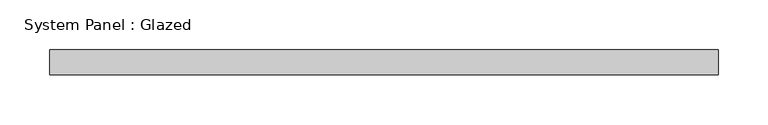
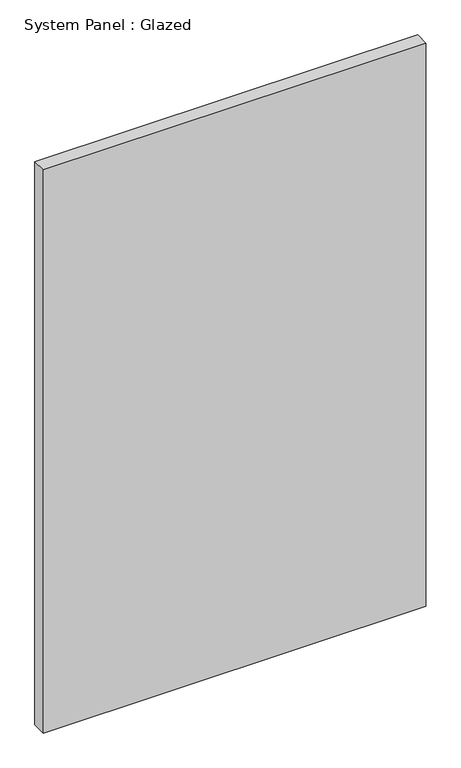
"""IFC4 building model written with IfcOpenShell, lengths in millimetres: plate geometry, System Panel : Glazed."""

from ifc_helpers import new_model, si_unit, origin, origin_with_axes, place, context, project, spatial, polyline, outline, extrude, source, transform, mapped, element, save


def system_panel_glazed_4f773535(model_context):
    return source(origin(), model_context, "Body", "SweptSolid", [
        extrude(outline(polyline([(336.55, 19.05), (-336.55, 19.05), (-336.55, 44.45), (336.55, 44.45), (336.55, 19.05)])), origin_with_axes(), (0.0, 0.0, 1.0), 1047.2243728),
    ])


if __name__ == "__main__":
    model = new_model("IFC4")
    model_context = context("Model", 3, world=origin())
    ifc_project = project(units=[si_unit("LENGTHUNIT", "METRE", prefix="MILLI")], contexts=[model_context])
    site = spatial("IfcSite", under=ifc_project)
    building = spatial("IfcBuilding", under=site)
    placement = place(None, origin())
    system_panel_glazed_shape = system_panel_glazed_4f773535(model_context)
    element("IfcPlate", 1, ObjectType="System Panel : Glazed", at=placement, inside=building, context=model_context, shape_type="MappedRepresentation", body=[
        mapped(system_panel_glazed_shape, transform((0.0, 0.0, 0.0), x_axis=(1.0, 0.0, 0.0), y_axis=(0.0, 1.0, 0.0), z_axis=(0.0, 0.0, 1.0))),
    ])
    save(model, "model.ifc")

# Revit data of these elements
# Type "System Panel : Glazed"
#   Construction Type Id = "GSP4R"
#   Analytic Construction = "1/8 in Pilkington single glazing"
#   Visual Light Transmittance = 0.9
#   Solar Heat Gain Coefficient = 0.86
#   Heat Transfer Coefficient (U) = 1.18115 BTU/(h·ft²·°F)
#   Define Thermal Properties by = 1
# Element 1 (IfcPlate, "System Panel : Glazed")
#   Materials on its faces: "Glass"
# Materials
#   "Glass": class "Glass", colour RGB 0 128 192, transparency 0.75, Description = "Soda Lime Glass", Cost = 0
